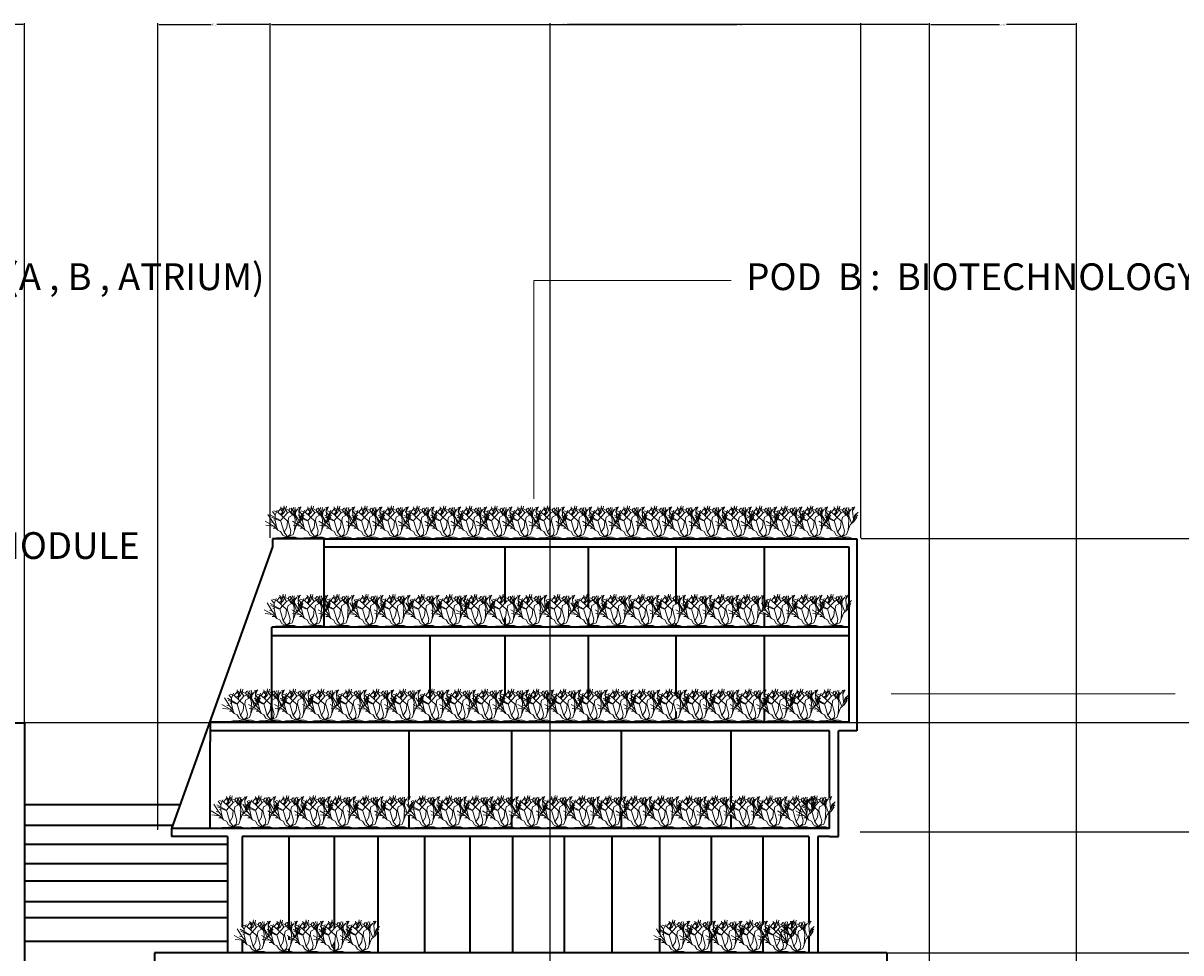
# Model space of a CAD drawing. Units: inches. Extents: x -160 to 434, y -145 to 103.
# Tile 6 of 7: x 107 to 262, y -22 to 103. Entities that reach past the tile are written whole.
import ezdxf

# ---------------------------------------------------------------- set-up
doc = ezdxf.new("R2010")
doc.units = ezdxf.units.IN
doc.header["$MEASUREMENT"] = 0
for name, color, linetype, lineweight in [('A-ANNO-DIMS', 2, 'Continuous', 18), ('A-ANNO-SYMB', 2, 'Continuous', 13), ('A-ANNO-TEXT', 3, 'Continuous', 18), ('A-ELEV', 7, 'Continuous', 35), ('L-PLNT', 3, 'Continuous', 13)]:
    doc.layers.add(name, color=color, linetype=linetype, lineweight=lineweight)
doc.styles.get("Standard").update_dxf_attribs({"font": 'arial.ttf'})
doc.dimstyles.get("Standard").update_dxf_attribs({"dimtxt": 0.18, "dimasz": 0.18, "dimexe": 0.18, "dimexo": 0.0625, "dimgap": 0.09, "dimtad": 0, "dimtih": 1, "dimtoh": 1, "dimdec": 4, "dimzin": 0, "dimdsep": 46, "dimtxsty": 'Standard', "dimcen": 0.09, "dimadec": 0, "dimazin": 0, "dimtfac": 1, "dimtdec": 4, "dimtofl": 0, "dimtmove": 0, "dimatfit": 3, "dimfxl": 1, "dimtolj": 1, "dimtzin": 0, "dimarcsym": 0})

# ---------------------------------------------------------------- blocks, each defined once
blk = doc.blocks.new('*U5')
for p, q in [((-18.24, 11.04), (-21.755, 16.655)), ((-12.96, 12.48), (-19.68, 16.32)), ((-16.8, 16.32), (-18.72, 18.72)), ((-14.88, 18.24), (-17.76, 19.2)), ((-16.8, 16.32), (-15.36, 19.68)), ((-16.8, 12.48), (-16.8, 16.32)), ((-14.88, 18.24), (-12.96, 20.64)), ((-8.16, 12), (-14.88, 18.24)), ((-13.325, 16.724), (-11.433, 18.289)), ((-12.96, 12.48), (-8.16, 17.76)), ((-12.471, 19.775), (-12.898, 22.044)), ((-11.677, 19.071), (-12.471, 19.775)), ((-11.28, 19.619), (-12.104, 21.184)), ((-12.043, 15.628), (-11.921, 18.836)), ((-11.982, 16.802), (-10.579, 18.054)), ((-11.921, 18.836), (-10.64, 20.401)), ((-11.433, 18.289), (-10.457, 22.749)), ((-10.579, 18.054), (-9.846, 19.697)), ((-8.16, 17.76), (-10.56, 21.6)), ((-9.48, 19.775), (-8.992, 22.592)), ((-7.2, 19.68), (-8.64, 20.16)), ((-8.16, 17.76), (-5.28, 19.2)), ((-7.2, 19.68), (-6.24, 21.12)), ((-4.8, 16.32), (-7.2, 19.68)), ((-7.2, 14.88), (-3.84, 16.8)), ((-5.086, 17.741), (-5.513, 21.34)), ((-5.28, 19.2), (-3.84, 21.6)), ((-3.377, 15.315), (-5.086, 17.819)), ((-2.88, 12.96), (-4.32, 19.68)), ((-3.84, 16.8), (-0.96, 20.64)), ((-3.377, 18.602), (-2.888, 21.575)), ((-2.766, 16.802), (-3.377, 18.602)), ((-2.88, 15.84), (-2.4, 20.16)), ((-0.508, 21.888), (-0.081, 20.558)), ((-0.203, 19.149), (0.102, 21.34)), ((0.346, 13.203), (-0.203, 19.149)), ((-0.142, 19.384), (0.59, 20.401)), ((-0.02, 20.01), (0.896, 21.105)), ((0.041, 20.714), (1.384, 22.044)), ((0.102, 21.34), (0.835, 21.888)), ((0.346, 13.203), (1.323, 16.254)), ((1.323, 16.254), (3.642, 18.289)), ((1.44, 15.36), (2.88, 17.28)), ((2.4, 15.36), (3.36, 16.32)), ((-17.76, 8.64), (-23.663, 11.961)), ((-17.76, 8.64), (-23.128, 9.222)), ((-18.24, 11.04), (-20.16, 11.52)), ((-13.92, 12.48), (-19.2, 14.88)), ((-15.84, 8.16), (-18.24, 11.04)), ((-16.8, 12.48), (-17.76, 12.96)), ((-14.88, 5.76), (-17.76, 8.64)), ((-15.84, 8.16), (-16.8, 12.48)), ((-14.88, 5.76), (-15.84, 8.16)), ((-12.96, 12.48), (-13.92, 12.48)), ((-10.56, 4.32), (-12.96, 12.48)), ((-8.64, 7.68), (-8.16, 12)), ((-7.68, 12.48), (-7.2, 14.88)), ((-6.72, 8.64), (-7.68, 12.48)), ((-5.76, 5.28), (-6.72, 8.64)), ((-4.32, 2.88), (-1.92, 9.6)), ((-3.36, 5.28), (-2.88, 12.96)), ((-0.96, 10.56), (-2.88, 15.84)), ((-1.92, 9.6), (0.96, 12)), ((-0.48, 10.8), (0.346, 13.203)), ((0.96, 12), (1.44, 15.36)), ((0.96, 12), (2.88, 14.88)), ((1.92, 13.44), (2.4, 15.36)), ((-16.32, 7.2), (-18.24, 7.2)), ((-15.84, 0.48), (-17.76, 0)), ((-13.44, 0.48), (-15.84, 0.48)), ((-12.96, 4.8), (-14.88, 5.76)), ((-9.6, 0.96), (-13.44, 0.48)), ((-11.52, 2.4), (-12.96, 4.8)), ((-9.6, 0.96), (-12.96, 0)), ((-8.64, 0.96), (-11.52, 2.4)), ((-10.56, 4.32), (-8.64, 7.68)), ((-8.64, 1.92), (-10.56, 4.32)), ((-9.6, 0.96), (-7.68, 0.96)), ((-8.64, 0.96), (-4.32, 2.88)), ((-8.64, 0.96), (-6.24, 2.88)), ((-8.64, 0.96), (-8.64, 1.92)), ((-8.64, 0.96), (-2.88, 0.96)), ((-7.68, 0.96), (-6.24, 0.48)), ((-6.24, 2.88), (-5.76, 5.28)), ((-6.24, 0.48), (-3.36, 0)), ((-2.88, 0.96), (0, 0))]:
    blk.add_line(p, q)
blk = doc.blocks.new('*D28')
at = {"layer": 'A-ANNO-DIMS', "color": 0, "lineweight": -2, "transparency": 16777216}
for p, q in [((78.69, 9.01), (78.69, 102.5)), ((78.87, 102.32), (92.58, 102.32)), ((107.09, 102.32), (93.38, 102.32)), ((107.27, 9.01), (107.27, 102.5))]:
    blk.add_line(p, q, dxfattribs=at)
at = {"layer": 'A-ANNO-DIMS', "color": 0, "transparency": 16777216}
for points in [[(78.87, 102.35), (78.87, 102.29), (78.69, 102.32)], [(107.09, 102.35), (107.09, 102.29), (107.27, 102.32)]]:
    blk.add_solid(points, dxfattribs=at)
at = {"layer": 'Defpoints', "color": 0, "transparency": 16777216}
for p in [(107.27, 102.32), (78.69, 8.95), (107.27, 8.95)]:
    blk.add_point(p, dxfattribs=at)
at = {"layer": 'A-ANNO-DIMS', "color": 0, "transparency": 16777216, "insert": (92.98, 102.32), "char_height": 0.18, "attachment_point": 5}
blk.add_mtext('\\A1;28.58', dxfattribs=at)
blk = doc.blocks.new('*D31')
at = {"layer": 'A-ANNO-DIMS', "color": 0, "lineweight": -2, "transparency": 16777216}
for p, q in [((107.33, 8.95), (433.98, 8.95)), ((433.8, 8.77), (433.8, -23.43)), ((433.8, -55.99), (433.8, -23.79)), ((107.33, -56.17), (433.98, -56.17))]:
    blk.add_line(p, q, dxfattribs=at)
at = {"layer": 'A-ANNO-DIMS', "color": 0, "transparency": 16777216}
for points in [[(433.77, 8.77), (433.83, 8.77), (433.8, 8.95)], [(433.77, -55.99), (433.83, -55.99), (433.8, -56.17)]]:
    blk.add_solid(points, dxfattribs=at)
at = {"layer": 'Defpoints', "color": 0, "transparency": 16777216}
for p in [(107.27, 8.95), (107.27, -56.17), (433.8, -56.17)]:
    blk.add_point(p, dxfattribs=at)
at = {"layer": 'A-ANNO-DIMS', "color": 0, "transparency": 16777216, "insert": (433.8, -23.61), "char_height": 0.18, "attachment_point": 5}
blk.add_mtext('\\A1;65.11', dxfattribs=at)
blk = doc.blocks.new('*D38')
at = {"layer": 'A-ANNO-DIMS', "color": 0, "lineweight": -2, "transparency": 16777216}
for p, q in [((140.1, 33.66), (140.1, 102.5)), ((140.28, 102.32), (179.18, 102.32)), ((218.87, 102.32), (179.97, 102.32)), ((219.05, 33.63), (219.05, 102.5))]:
    blk.add_line(p, q, dxfattribs=at)
at = {"layer": 'A-ANNO-DIMS', "color": 0, "transparency": 16777216}
for points in [[(140.28, 102.35), (140.28, 102.29), (140.1, 102.32)], [(218.87, 102.35), (218.87, 102.29), (219.05, 102.32)]]:
    blk.add_solid(points, dxfattribs=at)
at = {"layer": 'Defpoints', "color": 0, "transparency": 16777216}
for p in [(219.05, 102.32), (140.1, 33.59), (219.05, 33.57)]:
    blk.add_point(p, dxfattribs=at)
at = {"layer": 'A-ANNO-DIMS', "color": 0, "transparency": 16777216, "insert": (179.57, 102.32), "char_height": 0.18, "attachment_point": 5}
blk.add_mtext('\\A1;78.95', dxfattribs=at)
blk = doc.blocks.new('*D39')
at = {"layer": 'A-ANNO-DIMS', "color": 0, "lineweight": -2, "transparency": 16777216}
for p, q in [((125.09, -5.39), (125.09, 102.5)), ((125.27, 102.32), (132.22, 102.32)), ((139.92, 102.32), (132.96, 102.32)), ((140.1, 33.66), (140.1, 102.5))]:
    blk.add_line(p, q, dxfattribs=at)
at = {"layer": 'A-ANNO-DIMS', "color": 0, "transparency": 16777216}
for points in [[(125.27, 102.35), (125.27, 102.29), (125.09, 102.32)], [(139.92, 102.35), (139.92, 102.29), (140.1, 102.32)]]:
    blk.add_solid(points, dxfattribs=at)
at = {"layer": 'Defpoints', "color": 0, "transparency": 16777216}
for p in [(140.1, 102.32), (140.1, 33.59), (125.09, -5.45)]:
    blk.add_point(p, dxfattribs=at)
at = {"layer": 'A-ANNO-DIMS', "color": 0, "transparency": 16777216, "insert": (132.59, 102.32), "char_height": 0.18, "attachment_point": 5}
blk.add_mtext('\\A1;15.01', dxfattribs=at)
blk = doc.blocks.new('*D40')
at = {"layer": 'A-ANNO-DIMS', "color": 0, "lineweight": -2, "transparency": 16777216}
for p, q in [((219.11, 33.57), (433.98, 33.57)), ((433.8, 33.39), (433.8, 14.15)), ((433.8, -5.46), (433.8, 13.79)), ((218.99, -5.64), (433.98, -5.64))]:
    blk.add_line(p, q, dxfattribs=at)
at = {"layer": 'A-ANNO-DIMS', "color": 0, "transparency": 16777216}
for points in [[(433.77, 33.39), (433.83, 33.39), (433.8, 33.57)], [(433.77, -5.46), (433.83, -5.46), (433.8, -5.64)]]:
    blk.add_solid(points, dxfattribs=at)
at = {"layer": 'Defpoints', "color": 0, "transparency": 16777216}
for p in [(219.05, 33.57), (218.92, -5.64), (433.8, -5.64)]:
    blk.add_point(p, dxfattribs=at)
at = {"layer": 'A-ANNO-DIMS', "color": 0, "transparency": 16777216, "insert": (433.8, 13.97), "char_height": 0.18, "attachment_point": 5}
blk.add_mtext('\\A1;39.206', dxfattribs=at)
blk = doc.blocks.new('*D43')
at = {"layer": 'A-ANNO-DIMS', "color": 0, "lineweight": -2, "transparency": 16777216}
for p, q in [((222.5, -5.64), (433.98, -5.64)), ((433.8, -5.82), (433.8, -13.56)), ((433.8, -21.66), (433.8, -13.92)), ((222.59, -21.84), (433.98, -21.84))]:
    blk.add_line(p, q, dxfattribs=at)
at = {"layer": 'A-ANNO-DIMS', "color": 0, "transparency": 16777216}
for points in [[(433.77, -5.82), (433.83, -5.82), (433.8, -5.64)], [(433.77, -21.66), (433.83, -21.66), (433.8, -21.84)]]:
    blk.add_solid(points, dxfattribs=at)
at = {"layer": 'Defpoints', "color": 0, "transparency": 16777216}
for p in [(222.44, -5.64), (222.53, -21.84), (433.8, -21.84)]:
    blk.add_point(p, dxfattribs=at)
at = {"layer": 'A-ANNO-DIMS', "color": 0, "transparency": 16777216, "insert": (433.8, -13.74), "char_height": 0.18, "attachment_point": 5}
blk.add_mtext('\\A1;16.204', dxfattribs=at)
blk = doc.blocks.new('*D44')
at = {"layer": 'A-ANNO-DIMS', "color": 0, "lineweight": -2, "transparency": 16777216}
for p, q in [((177.54, -46.95), (177.54, 102.5)), ((177.72, 102.32), (202.52, 102.32)), ((228.07, 102.32), (203.27, 102.32)), ((228.25, -46.95), (228.25, 102.5))]:
    blk.add_line(p, q, dxfattribs=at)
at = {"layer": 'A-ANNO-DIMS', "color": 0, "transparency": 16777216}
for points in [[(177.72, 102.35), (177.72, 102.29), (177.54, 102.32)], [(228.07, 102.35), (228.07, 102.29), (228.25, 102.32)]]:
    blk.add_solid(points, dxfattribs=at)
at = {"layer": 'Defpoints', "color": 0, "transparency": 16777216}
for p in [(228.25, 102.32), (177.54, -47.01), (228.25, -47.01)]:
    blk.add_point(p, dxfattribs=at)
at = {"layer": 'A-ANNO-DIMS', "color": 0, "transparency": 16777216, "insert": (202.89, 102.32), "char_height": 0.18, "attachment_point": 5}
blk.add_mtext('\\A1;50.71', dxfattribs=at)
blk = doc.blocks.new('*D48')
at = {"layer": 'A-ANNO-DIMS', "color": 0, "lineweight": -2, "transparency": 16777216}
for p, q in [((228.25, -46.95), (228.25, 102.5)), ((228.43, 102.32), (237.61, 102.32)), ((247.69, 102.32), (238.52, 102.32)), ((247.87, -68.35), (247.87, 102.5))]:
    blk.add_line(p, q, dxfattribs=at)
at = {"layer": 'A-ANNO-DIMS', "color": 0, "transparency": 16777216}
for points in [[(228.43, 102.35), (228.43, 102.29), (228.25, 102.32)], [(247.69, 102.35), (247.69, 102.29), (247.87, 102.32)]]:
    blk.add_solid(points, dxfattribs=at)
at = {"layer": 'Defpoints', "color": 0, "transparency": 16777216}
for p in [(247.87, 102.32), (228.25, -47.01), (247.87, -68.41)]:
    blk.add_point(p, dxfattribs=at)
at = {"layer": 'A-ANNO-DIMS', "color": 0, "transparency": 16777216, "insert": (238.06, 102.32), "char_height": 0.18, "attachment_point": 5}
blk.add_mtext('\\A1;19.626', dxfattribs=at)

msp = doc.modelspace()

# ---------------------------------------------------------------- linework, layer by layer
at = {"layer": 'A-ANNO-SYMB'}
for p, q in [((175.3429, 38.8704), (175.3429, 68.0806)), ((175.3429, 68.0806), (201.7469, 68.0806)), ((223.1294, 12.781), (246.4868, 12.781)), ((246.4868, 12.781), (261.0586, 12.781))]:
    msp.add_line(p, q, dxfattribs=at)
at = {"layer": 'A-ELEV'}
for p, q in [((147.3166, 33.5292), (140.4174, 33.5292)), ((140.4174, 33.5292), (140.4174, 32.4575)), ((147.3166, 33.5292), (218.5191, 33.5292)), ((147.3166, 21.739), (147.3166, 33.5292)), ((218.5191, 33.5292), (218.5191, 18.0294)), ((140.4174, 32.4575), (126.9245, -5.216)), ((147.3166, 32.4575), (217.4461, 32.4575)), ((171.4641, 32.4575), (171.4641, 24.9055)), ((182.6113, 32.4575), (182.6113, 24.359)), ((194.3158, 32.4575), (194.3158, 24.8106)), ((206.1596, 32.4575), (206.1596, 24.1814)), ((217.4461, 32.4575), (217.4461, 18.0294)), ((206.1596, 23.6358), (206.1596, 21.739)), ((217.4461, 21.739), (140.3239, 21.739)), ((140.3239, 9.0255), (140.3239, 21.739)), ((171.4641, 22.9704), (171.4641, 21.739)), ((182.6113, 22.8394), (182.6113, 21.739)), ((194.3158, 22.2132), (194.3158, 21.739)), ((217.4461, 20.5698), (140.3239, 20.5698)), ((161.4317, 20.5698), (161.4317, 18.0294)), ((171.4641, 20.5698), (171.4641, 18.0294)), ((182.6113, 20.5698), (182.6113, 18.0294)), ((194.3158, 20.5698), (194.3158, 18.0294)), ((206.1596, 20.5698), (206.1596, 18.0294)), ((161.4317, 18.0294), (161.4317, 12.0952)), ((171.4641, 18.0294), (171.4641, 12.5032)), ((182.6113, 18.0294), (182.6113, 12.0704)), ((194.3158, 18.0294), (194.3158, 12.6103)), ((206.1596, 18.0294), (206.1596, 12.5798)), ((217.4461, 18.0294), (217.4461, 9.0255)), ((218.5191, 18.0294), (218.5191, 7.8563)), ((171.4641, 11.7422), (171.4641, 11.6058)), ((206.1596, 12.2016), (206.1596, 11.2103)), ((161.4317, 9.7294), (161.4317, 9.0255)), ((171.4641, 10.3931), (171.4641, 10.2729)), ((182.6113, 9.6849), (182.6113, 9.0255)), ((194.3158, 10.4195), (194.3158, 9.6444)), ((206.1596, 10.8029), (206.1596, 9.0255)), ((78.691, 8.9457), (107.2684, 8.9457)), ((107.2684, 8.9457), (107.2684, -38.311)), ((138.3454, 9.0255), (132.0251, 9.0255)), ((132.0683, 9.0255), (132.0683, 6.4296)), ((214.894, 7.8563), (132.0683, 7.8563)), ((217.4461, 9.0255), (138.3454, 9.0255)), ((158.7053, -1.2555), (158.7053, 7.8563)), ((171.4641, 9.177), (171.4641, 9.0255)), ((172.4065, -2.3438), (172.4065, 7.8563)), ((187.0765, -1.4314), (187.0765, 7.8563)), ((194.3158, 9.2693), (194.3158, 9.0255)), ((201.7464, -1.6166), (201.7464, 7.8563)), ((214.894, -1.1189), (214.894, 7.8563)), ((218.5191, 7.8563), (216.0869, 7.8563)), ((216.0869, -6.2877), (216.0869, 7.8563)), ((132.0683, -5.216), (132.0683, 6.4296)), ((107.2684, -2.0014), (128.0758, -2.0014)), ((158.7053, -2.5191), (158.7053, -2.5115)), ((158.7053, -2.9599), (158.7053, -2.925)), ((187.0765, -2.6466), (187.0765, -2.597)), ((187.0765, -5.216), (187.0765, -2.9721)), ((201.7464, -3.0291), (201.7464, -2.1555)), ((214.894, -5.216), (214.894, -2.9505)), ((158.7053, -5.216), (158.7053, -3.4579)), ((172.4065, -5.216), (172.4065, -3.4231)), ((201.7464, -5.216), (201.7464, -3.423)), ((107.2684, -4.7649), (127.086, -4.7649)), ((128.0758, -5.216), (126.9245, -5.216)), ((126.9245, -5.216), (126.9245, -6.2877)), ((214.894, -5.216), (128.0758, -5.216)), ((107.2684, -7.3158), (134.424, -7.3158)), ((128.0758, -6.2877), (126.9245, -6.2877)), ((134.424, -6.2877), (128.0758, -6.2877)), ((134.424, -6.2877), (134.424, -21.8399)), ((137.8943, -6.2877), (136.3653, -6.2877)), ((136.3653, -6.2877), (136.3653, -18.3411)), ((212.0903, -6.2877), (137.8943, -6.2877)), ((142.5931, -6.2877), (142.5931, -18.6884)), ((148.6825, -6.2877), (148.6825, -18.5622)), ((154.4952, -6.2877), (154.4952, -18.5801)), ((160.723, -6.2877), (160.723, -21.8399)), ((166.8124, -6.2877), (166.8124, -21.8399)), ((172.4867, -6.2877), (172.4867, -21.8399)), ((179.4065, -6.2877), (179.4065, -21.8399)), ((185.7727, -6.2877), (185.7727, -21.8399)), ((192.1389, -6.2877), (192.1389, -19.2477)), ((199.0587, -6.2877), (199.0587, -18.0257)), ((205.9785, -6.2877), (205.9785, -18.0356)), ((212.0903, -6.2877), (212.0903, -17.7782)), ((214.894, -6.2877), (213.3013, -6.2877)), ((213.3013, -6.2877), (213.3013, -21.8399)), ((214.894, -6.2877), (216.0869, -6.2877)), ((107.2684, -9.8667), (134.424, -9.8667)), ((107.2684, -12.2051), (134.424, -12.2051)), ((107.2684, -14.9686), (134.424, -14.9686)), ((107.2684, -17.0943), (134.424, -17.0943)), ((136.3653, -20.1097), (136.3653, -21.8399)), ((142.5931, -19.6301), (142.5931, -20.0572)), ((154.4952, -19.0521), (154.4952, -19.2335)), ((154.4952, -19.0521), (154.4952, -21.8399)), ((160.723, -19.6124), (160.723, -21.8399)), ((172.4867, -19.3841), (172.4867, -19.4205)), ((179.4065, -19.3305), (179.4065, -19.4205)), ((185.7727, -19.0309), (185.7727, -19.6762)), ((185.7727, -20.0981), (185.7727, -21.8399)), ((192.1389, -19.6271), (192.1389, -19.6472)), ((192.1389, -19.8639), (192.1389, -21.8399)), ((199.0587, -19.4292), (199.0587, -21.8399)), ((205.9785, -19.1525), (205.9785, -19.4087)), ((205.9785, -19.6122), (205.9785, -21.8399)), ((212.0903, -19.603), (212.0903, -21.8399)), ((107.2684, -20.283), (134.424, -20.283)), ((142.5931, -21.3031), (142.5931, -21.8399)), ((148.6825, -20.4327), (148.6825, -21.8399)), ((166.8124, -20.3715), (166.8124, -21.8399)), ((172.4867, -20.866), (172.4867, -21.8399)), ((179.4065, -20.8191), (179.4065, -21.8399)), ((137.8943, -21.8399), (124.6537, -21.8399)), ((124.6537, -21.8399), (124.6537, -41.3403)), ((212.0903, -21.8399), (137.8943, -21.8399)), ((154.4952, -21.7394), (154.4952, -21.8399)), ((222.5284, -21.8399), (212.0903, -21.8399)), ((222.5284, -21.8399), (222.5284, -41.3403))]:
    msp.add_line(p, q, dxfattribs=at)

# ---------------------------------------------------------------- block references
at = {"layer": 'L-PLNT', "xscale": 0.1923638725067976, "yscale": 0.1923638725067976, "zscale": 0.1923638725067976}
for p in [(143.999, 33.5746), (147.6409, 33.5746), (151.1587, 33.5746), (154.8006, 33.5746), (158.3184, 33.5746), (161.7687, 33.5746), (165.321, 33.5746), (168.7974, 33.5746), (172.191, 33.5746), (175.7088, 33.5746), (179.1959, 33.5746), (182.8378, 33.5746), (186.397, 33.5746), (189.8734, 33.5746), (193.5232, 33.5746), (197.041, 33.5746), (200.6001, 33.5746), (204.2007, 33.5746), (207.563, 33.5746), (210.9566, 33.5746), (214.3916, 33.5746), (217.9921, 33.5746), (143.8784, 21.7559), (147.5448, 21.7559), (151.0779, 21.7559), (154.9443, 21.7559), (158.5441, 21.7559), (162.4105, 21.7559), (166.1435, 21.7559), (169.4766, 21.7559), (173.2764, 21.7559), (176.8095, 21.7559), (180.5653, 21.7559), (184.4983, 21.7559), (188.0981, 21.7559), (191.8312, 21.7559), (195.3643, 21.7559), (198.8973, 21.7559), (202.4971, 21.7559), (205.8969, 21.7559), (209.9632, 21.7559), (213.6297, 21.7559), (217.0961, 21.7559), (138.1772, 9.0847), (141.7579, 9.0847), (145.2282, 9.0847), (149.0013, 9.0847), (152.701, 9.0847), (156.3582, 9.0847), (159.9303, 9.0847), (163.7576, 9.0847), (167.2872, 9.0847), (170.8771, 9.0847), (174.4067, 9.0847), (177.7662, 9.0847), (181.3809, 9.0847), (184.9105, 9.0847), (188.3976, 9.0847), (191.9272, 9.0847), (195.515, 9.0847), (199.0021, 9.0847), (202.5317, 9.0847), (206.1463, 9.0847), (209.676, 9.0847), (213.0355, 9.0847), (216.6927, 9.0847), (136.7527, -5.1654), (140.6198, -5.1654), (144.3447, -5.1654), (147.8984, -5.1654), (151.2808, -5.1654), (154.9629, -5.1654), (158.6022, -5.1654), (162.5412, -5.1654), (166.0948, -5.1654), (169.6485, -5.1654), (173.0309, -5.1654), (176.5633, -5.1654), (180.2026, -5.1654), (183.8847, -5.1654), (187.4384, -5.1654), (190.8636, -5.1654), (194.4601, -5.1654), (198.185, -5.1654), (201.6531, -5.1654), (205.3057, -5.1654), (208.945, -5.1654), (212.4558, -5.1654), (214.9391, -5.1654), (139.8696, -21.8212), (143.5048, -21.8212), (146.95, -21.8212), (150.3953, -21.8212), (154.0033, -21.8212), (195.9292, -21.8212), (199.3745, -21.8212), (202.9107, -21.8212), (206.3018, -21.8212), (209.8284, -21.8212), (212.1343, -21.8212)]:
    msp.add_blockref('*U5', p, dxfattribs=at)

# ---------------------------------------------------------------- texts
at = {"layer": 'A-ANNO-TEXT'}
for s, p in [('MODULAR   PODS  (A , B , ATRIUM)', (63.2171, 66.798)), ('POD  B :  BIOTECHNOLOGY  AND   GENOMICS', (203.7515, 66.798)), ('SPINE   ATRIUM  MODULE', (65.4677, 30.8438))]:
    msp.add_text(s, height=3.579169, dxfattribs=at).set_placement(p)

# ---------------------------------------------------------------- dimensions: what is measured, and where the dimension line sits
at = {"layer": 'A-ANNO-DIMS'}
for base, p1, p2, override, picture, middle in [((107.2684, 102.3218), (78.691, 8.9457), (107.2684, 8.9457), {"dimdec": 2, "dimlfac": 1, "dimrnd": 0, "dimzin": 0, "dimdsep": 46, "dimlunit": 2}, '*D28', (92.9797, 102.3218)), ((140.0969, 102.3218), (125.0856, -5.4476), (140.0969, 33.5927), {"dimdec": 2, "dimlfac": 1, "dimrnd": 0, "dimzin": 0, "dimdsep": 46, "dimlunit": 2}, '*D39', (132.5912, 102.3218)), ((219.0478, 102.3218), (140.0969, 33.5927), (219.0478, 33.5699), {"dimdec": 2, "dimlfac": 1, "dimrnd": 0, "dimzin": 0, "dimdsep": 46, "dimlunit": 2}, '*D38', (179.5723, 102.3218)), ((228.249, 102.3218), (177.5358, -47.0121), (228.249, -47.0121), {"dimdec": 2, "dimlfac": 1, "dimrnd": 0, "dimzin": 0, "dimdsep": 46, "dimlunit": 2}, '*D44', (202.8924, 102.3218)), ((247.8746, 102.3218), (228.249, -47.0121), (247.8746, -68.412), {"dimdec": 3, "dimlfac": 1, "dimrnd": 0, "dimzin": 0, "dimdsep": 46, "dimlunit": 2}, '*D48', (238.0618, 102.3218))]:
    dim = msp.add_linear_dim(base=base, p1=p1, p2=p2, dimstyle='Standard', override=override, dxfattribs=at)
    dim.commit()
    dim.dimension.update_dxf_attribs({"geometry": picture, "text_midpoint": middle})
for base, p1, p2, override, picture, middle in [((433.7977, -5.6358), (219.0478, 33.5699), (218.9244, -5.6358), {"dimdec": 3, "dimlfac": 1, "dimrnd": 0, "dimzin": 0, "dimdsep": 46, "dimlunit": 2}, '*D40', (433.7977, 13.9671)), ((433.7977, -56.1669), (107.2684, 8.9457), (107.2684, -56.1669), {"dimdec": 2, "dimlfac": 1, "dimrnd": 0, "dimzin": 0, "dimdsep": 46, "dimlunit": 2}, '*D31', (433.7977, -23.6106)), ((433.7977, -21.8399), (222.4353, -5.6358), (222.5284, -21.8399), {"dimdec": 3, "dimlfac": 1, "dimrnd": 0, "dimzin": 0, "dimdsep": 46, "dimlunit": 2}, '*D43', (433.7977, -13.7378))]:
    dim = msp.add_linear_dim(base=base, p1=p1, p2=p2, angle=90, dimstyle='Standard', override=override, dxfattribs=at)
    dim.commit()
    dim.dimension.update_dxf_attribs({"geometry": picture, "text_midpoint": middle})

doc.saveas('drawing.dxf')
